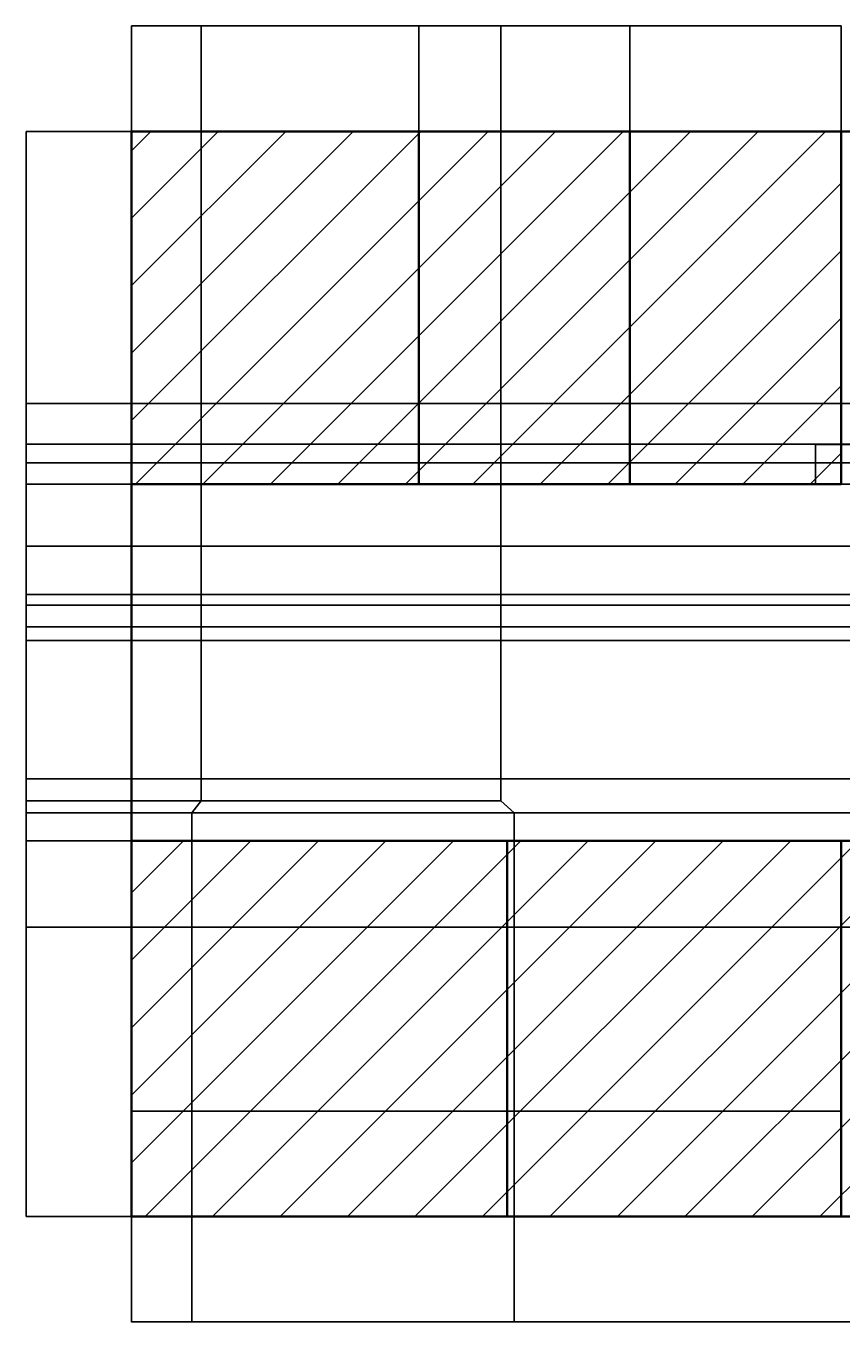
# Model space of a CAD drawing. Units: millimetres. Extents: x 2212 to 7718, y 1114 to 4219.
# Tile 1 of 5: x 2212 to 4165, y 1114 to 4219. Entities that reach past the tile are written whole.
import ezdxf

# ---------------------------------------------------------------- set-up
doc = ezdxf.new("R2010")
doc.units = ezdxf.units.MM
for name, color, linetype, lineweight in [('A-ANNO-DIMS', 2, 'Continuous', 18), ('A-ELEV-PATT', 8, 'Continuous', 13), ('A-FLOR-FIXT', 3, 'Continuous', 25), ('A-FURN', 7, 'Continuous', 35), ('A-FURN-CTOP', 6, 'Continuous', 25)]:
    doc.layers.add(name, color=color, linetype=linetype, lineweight=lineweight)
doc.styles.get("Standard").update_dxf_attribs({"font": 'arial.ttf'})
doc.dimstyles.get("Standard").update_dxf_attribs({"dimtxt": 0.18, "dimasz": 0.18, "dimexe": 0.18, "dimexo": 0.0625, "dimgap": 0.09, "dimtad": 0, "dimtih": 1, "dimtoh": 1, "dimdec": 4, "dimzin": 0, "dimdsep": 46, "dimtxsty": 'Standard', "dimcen": 0.09, "dimadec": 0, "dimazin": 0, "dimtfac": 1, "dimtdec": 4, "dimtofl": 0, "dimtmove": 0, "dimatfit": 3, "dimfxl": 1, "dimtolj": 1, "dimtzin": 0, "dimarcsym": 0})

# ---------------------------------------------------------------- blocks, each defined once
blk = doc.blocks.new('*D1')
at = {"layer": 'A-ANNO-DIMS', "color": 0, "lineweight": -2, "transparency": 16777216}
for p, q in [((2465.1, 3966.2), (2465.1, 4218.9)), ((2465.3, 4218.7), (2808.9, 4218.7)), ((3153.3, 4218.7), (2809.7, 4218.7)), ((3153.5, 3966.2), (3153.5, 4218.9))]:
    blk.add_line(p, q, dxfattribs=at)
at = {"layer": 'A-ANNO-DIMS', "color": 0, "transparency": 16777216}
for points in [[(2465.3, 4218.7), (2465.3, 4218.7), (2465.1, 4218.7)], [(3153.3, 4218.7), (3153.3, 4218.7), (3153.5, 4218.7)]]:
    blk.add_solid(points, dxfattribs=at)
at = {"layer": 'Defpoints', "color": 0, "transparency": 16777216}
for p in [(3153.5, 4218.7), (2465.1, 3966.2), (3153.5, 3966.2)]:
    blk.add_point(p, dxfattribs=at)
at = {"layer": 'A-ANNO-DIMS', "color": 0, "transparency": 16777216, "insert": (2809.3, 4218.7), "char_height": 0.18, "attachment_point": 5}
blk.add_mtext('\\A1;688.3', dxfattribs=at)
blk = doc.blocks.new('*D2')
at = {"layer": 'A-ANNO-DIMS', "color": 0, "lineweight": -2, "transparency": 16777216}
for p, q in [((3153.5, 3966.2), (3153.5, 4218.9)), ((3153.6, 4218.7), (3406, 4218.7)), ((3659.1, 4218.7), (3406.8, 4218.7)), ((3659.3, 3966.2), (3659.3, 4218.9))]:
    blk.add_line(p, q, dxfattribs=at)
at = {"layer": 'A-ANNO-DIMS', "color": 0, "transparency": 16777216}
for points in [[(3153.6, 4218.7), (3153.6, 4218.7), (3153.5, 4218.7)], [(3659.1, 4218.7), (3659.1, 4218.7), (3659.3, 4218.7)]]:
    blk.add_solid(points, dxfattribs=at)
at = {"layer": 'Defpoints', "color": 0, "transparency": 16777216}
for p in [(3659.3, 4218.7), (3153.5, 3966.2), (3659.3, 3966.2)]:
    blk.add_point(p, dxfattribs=at)
at = {"layer": 'A-ANNO-DIMS', "color": 0, "transparency": 16777216, "insert": (3406.4, 4218.7), "char_height": 0.18, "attachment_point": 5}
blk.add_mtext('\\A1;505.8', dxfattribs=at)
blk = doc.blocks.new('*D3')
at = {"layer": 'A-ANNO-DIMS', "color": 0, "lineweight": -2, "transparency": 16777216}
for p, q in [((3659.3, 3966.2), (3659.3, 4218.9)), ((3659.5, 4218.7), (3911.8, 4218.7)), ((4165, 4218.7), (3912.6, 4218.7)), ((4165.1, 3966.2), (4165.1, 4218.9))]:
    blk.add_line(p, q, dxfattribs=at)
at = {"layer": 'A-ANNO-DIMS', "color": 0, "transparency": 16777216}
for points in [[(3659.5, 4218.7), (3659.5, 4218.7), (3659.3, 4218.7)], [(4165, 4218.7), (4165, 4218.7), (4165.1, 4218.7)]]:
    blk.add_solid(points, dxfattribs=at)
at = {"layer": 'Defpoints', "color": 0, "transparency": 16777216}
for p in [(4165.1, 4218.7), (3659.3, 3966.2), (4165.1, 3966.2)]:
    blk.add_point(p, dxfattribs=at)
at = {"layer": 'A-ANNO-DIMS', "color": 0, "transparency": 16777216, "insert": (3912.2, 4218.7), "char_height": 0.18, "attachment_point": 5}
blk.add_mtext('\\A1;505.8', dxfattribs=at)
blk = doc.blocks.new('*D12')
at = {"layer": 'A-ANNO-DIMS', "color": 0, "lineweight": -2, "transparency": 16777216}
for p, q in [((4356.7, 3216.4), (4104, 3216.4)), ((4104.2, 3216.2), (4104.2, 3169)), ((4104.2, 3121.5), (4104.2, 3168.7)), ((4356.7, 3121.3), (4104, 3121.3))]:
    blk.add_line(p, q, dxfattribs=at)
at = {"layer": 'A-ANNO-DIMS', "color": 0, "transparency": 16777216}
for points in [[(4104.2, 3216.2), (4104.2, 3216.2), (4104.2, 3216.4)], [(4104.2, 3121.5), (4104.2, 3121.5), (4104.2, 3121.3)]]:
    blk.add_solid(points, dxfattribs=at)
at = {"layer": 'Defpoints', "color": 0, "transparency": 16777216}
for p in [(4104.2, 3216.4), (4356.7, 3216.4), (4356.7, 3121.3)]:
    blk.add_point(p, dxfattribs=at)
at = {"layer": 'A-ANNO-DIMS', "color": 0, "transparency": 16777216, "insert": (4104.2, 3168.9), "char_height": 0.18, "attachment_point": 5}
blk.add_mtext('\\A1;95.06', dxfattribs=at)
blk = doc.blocks.new('*D13')
at = {"layer": 'A-ANNO-DIMS', "color": 0, "lineweight": -2, "transparency": 16777216}
for p, q in [((2465.1, 1366.2), (2465.1, 1618.9)), ((2465.3, 1618.7), (2914.9, 1618.7)), ((3365, 1618.7), (2915.4, 1618.7)), ((3365.1, 1366.2), (3365.1, 1618.9))]:
    blk.add_line(p, q, dxfattribs=at)
at = {"layer": 'A-ANNO-DIMS', "color": 0, "transparency": 16777216}
for points in [[(2465.3, 1618.7), (2465.3, 1618.7), (2465.1, 1618.7)], [(3365, 1618.7), (3365, 1618.7), (3365.1, 1618.7)]]:
    blk.add_solid(points, dxfattribs=at)
at = {"layer": 'Defpoints', "color": 0, "transparency": 16777216}
for p in [(3365.1, 1618.7), (2465.1, 1366.2), (3365.1, 1366.2)]:
    blk.add_point(p, dxfattribs=at)
at = {"layer": 'A-ANNO-DIMS', "color": 0, "transparency": 16777216, "insert": (2915.1, 1618.7), "char_height": 0.18, "attachment_point": 5}
blk.add_mtext('\\A1;900', dxfattribs=at)
blk = doc.blocks.new('*D14')
at = {"layer": 'A-ANNO-DIMS', "color": 0, "lineweight": -2, "transparency": 16777216}
for p, q in [((3365.1, 1366.2), (3365.1, 1618.9)), ((3365.3, 1618.7), (3764.9, 1618.7)), ((4165, 1618.7), (3765.4, 1618.7)), ((4165.1, 1366.2), (4165.1, 1618.9))]:
    blk.add_line(p, q, dxfattribs=at)
at = {"layer": 'A-ANNO-DIMS', "color": 0, "transparency": 16777216}
for points in [[(3365.3, 1618.7), (3365.3, 1618.7), (3365.1, 1618.7)], [(4165, 1618.7), (4165, 1618.7), (4165.1, 1618.7)]]:
    blk.add_solid(points, dxfattribs=at)
at = {"layer": 'Defpoints', "color": 0, "transparency": 16777216}
for p in [(4165.1, 1618.7), (3365.1, 1366.2), (4165.1, 1366.2)]:
    blk.add_point(p, dxfattribs=at)
at = {"layer": 'A-ANNO-DIMS', "color": 0, "transparency": 16777216, "insert": (3765.1, 1618.7), "char_height": 0.18, "attachment_point": 5}
blk.add_mtext('\\A1;800', dxfattribs=at)
blk = doc.blocks.new('*D18')
at = {"layer": 'A-ANNO-DIMS', "color": 0, "lineweight": -2, "transparency": 16777216}
for p, q in [((2465.1, 1366.1), (2465.1, 1113.5)), ((7465.1, 1366.1), (7465.1, 1113.5)), ((2465.3, 1113.7), (4964.8, 1113.7)), ((7465, 1113.7), (4965.5, 1113.7))]:
    blk.add_line(p, q, dxfattribs=at)
at = {"layer": 'A-ANNO-DIMS', "color": 0, "transparency": 16777216}
for points in [[(2465.3, 1113.7), (2465.3, 1113.7), (2465.1, 1113.7)], [(7465, 1113.7), (7465, 1113.7), (7465.1, 1113.7)]]:
    blk.add_solid(points, dxfattribs=at)
at = {"layer": 'Defpoints', "color": 0, "transparency": 16777216}
for p in [(2465.1, 1366.2), (7465.1, 1366.2), (7465.1, 1113.7)]:
    blk.add_point(p, dxfattribs=at)
at = {"layer": 'A-ANNO-DIMS', "color": 0, "transparency": 16777216, "insert": (4965.1, 1113.7), "char_height": 0.18, "attachment_point": 5}
blk.add_mtext('\\A1;5000', dxfattribs=at)
blk = doc.blocks.new('*D19')
at = {"layer": 'A-ANNO-DIMS', "color": 0, "lineweight": -2, "transparency": 16777216}
for p, q in [((2465.1, 2266.4), (2212.5, 2266.4)), ((2212.6, 2266.2), (2212.6, 1816.5)), ((2212.6, 1366.4), (2212.6, 1816.1)), ((2465.1, 1366.2), (2212.5, 1366.2))]:
    blk.add_line(p, q, dxfattribs=at)
at = {"layer": 'A-ANNO-DIMS', "color": 0, "transparency": 16777216}
for points in [[(2212.6, 2266.2), (2212.7, 2266.2), (2212.6, 2266.4)], [(2212.6, 1366.4), (2212.7, 1366.4), (2212.6, 1366.2)]]:
    blk.add_solid(points, dxfattribs=at)
at = {"layer": 'Defpoints', "color": 0, "transparency": 16777216}
for p in [(2212.6, 2266.4), (2465.1, 2266.4), (2465.1, 1366.2)]:
    blk.add_point(p, dxfattribs=at)
at = {"layer": 'A-ANNO-DIMS', "color": 0, "transparency": 16777216, "insert": (2212.6, 1816.3), "char_height": 0.18, "attachment_point": 5}
blk.add_mtext('\\A1;900.2', dxfattribs=at)
blk = doc.blocks.new('*D20')
at = {"layer": 'A-ANNO-DIMS', "color": 0, "lineweight": -2, "transparency": 16777216}
for p, q in [((2465.1, 2333.4), (2212.5, 2333.4)), ((2212.6, 2333.2), (2212.6, 2300.1)), ((2212.6, 2266.6), (2212.6, 2299.7)), ((2465.1, 2266.4), (2212.5, 2266.4))]:
    blk.add_line(p, q, dxfattribs=at)
at = {"layer": 'A-ANNO-DIMS', "color": 0, "transparency": 16777216}
for points in [[(2212.6, 2333.2), (2212.7, 2333.2), (2212.6, 2333.4)], [(2212.6, 2266.6), (2212.7, 2266.6), (2212.6, 2266.4)]]:
    blk.add_solid(points, dxfattribs=at)
at = {"layer": 'Defpoints', "color": 0, "transparency": 16777216}
for p in [(2212.6, 2333.4), (2465.1, 2333.4), (2465.1, 2266.4)]:
    blk.add_point(p, dxfattribs=at)
at = {"layer": 'A-ANNO-DIMS', "color": 0, "transparency": 16777216, "insert": (2212.6, 2299.9), "char_height": 0.18, "attachment_point": 5}
blk.add_mtext('\\A1;66.97', dxfattribs=at)
blk = doc.blocks.new('*D21')
at = {"layer": 'A-ANNO-DIMS', "color": 0, "lineweight": -2, "transparency": 16777216}
for p, q in [((2465.1, 2414.8), (2212.5, 2414.8)), ((2212.6, 2414.6), (2212.6, 2374.3)), ((2212.6, 2333.5), (2212.6, 2373.9)), ((2465.1, 2333.4), (2212.5, 2333.4))]:
    blk.add_line(p, q, dxfattribs=at)
at = {"layer": 'A-ANNO-DIMS', "color": 0, "transparency": 16777216}
for points in [[(2212.6, 2414.6), (2212.7, 2414.6), (2212.6, 2414.8)], [(2212.6, 2333.5), (2212.7, 2333.5), (2212.6, 2333.4)]]:
    blk.add_solid(points, dxfattribs=at)
at = {"layer": 'Defpoints', "color": 0, "transparency": 16777216}
for p in [(2212.6, 2414.8), (2465.1, 2414.8), (2465.1, 2333.4)]:
    blk.add_point(p, dxfattribs=at)
at = {"layer": 'A-ANNO-DIMS', "color": 0, "transparency": 16777216, "insert": (2212.6, 2374.1), "char_height": 0.18, "attachment_point": 5}
blk.add_mtext('\\A1;81.45', dxfattribs=at)
blk = doc.blocks.new('*D22')
at = {"layer": 'A-ANNO-DIMS', "color": 0, "lineweight": -2, "transparency": 16777216}
for p, q in [((2465.1, 3121.3), (2212.5, 3121.3)), ((2212.6, 3121.2), (2212.6, 2768.3)), ((2212.6, 2415), (2212.6, 2767.9)), ((2465.1, 2414.8), (2212.5, 2414.8))]:
    blk.add_line(p, q, dxfattribs=at)
at = {"layer": 'A-ANNO-DIMS', "color": 0, "transparency": 16777216}
for points in [[(2212.6, 3121.2), (2212.7, 3121.2), (2212.6, 3121.3)], [(2212.6, 2415), (2212.7, 2415), (2212.6, 2414.8)]]:
    blk.add_solid(points, dxfattribs=at)
at = {"layer": 'Defpoints', "color": 0, "transparency": 16777216}
for p in [(2212.6, 3121.3), (2465.1, 3121.3), (2465.1, 2414.8)]:
    blk.add_point(p, dxfattribs=at)
at = {"layer": 'A-ANNO-DIMS', "color": 0, "transparency": 16777216, "insert": (2212.6, 2768.1), "char_height": 0.18, "attachment_point": 5}
blk.add_mtext('\\A1;706.5', dxfattribs=at)
blk = doc.blocks.new('*D23')
at = {"layer": 'A-ANNO-DIMS', "color": 0, "lineweight": -2, "transparency": 16777216}
for p, q in [((2465.1, 3966.2), (2212.5, 3966.2)), ((2212.6, 3966), (2212.6, 3543.9)), ((2212.6, 3121.5), (2212.6, 3543.6)), ((2465.1, 3121.3), (2212.5, 3121.3))]:
    blk.add_line(p, q, dxfattribs=at)
at = {"layer": 'A-ANNO-DIMS', "color": 0, "transparency": 16777216}
for points in [[(2212.6, 3966), (2212.7, 3966), (2212.6, 3966.2)], [(2212.6, 3121.5), (2212.7, 3121.5), (2212.6, 3121.3)]]:
    blk.add_solid(points, dxfattribs=at)
at = {"layer": 'Defpoints', "color": 0, "transparency": 16777216}
for p in [(2212.6, 3966.2), (2465.1, 3966.2), (2465.1, 3121.3)]:
    blk.add_point(p, dxfattribs=at)
at = {"layer": 'A-ANNO-DIMS', "color": 0, "transparency": 16777216, "insert": (2212.6, 3543.8), "char_height": 0.18, "attachment_point": 5}
blk.add_mtext('\\A1;844.8', dxfattribs=at)
blk = doc.blocks.new('*D27')
at = {"layer": 'A-ANNO-DIMS', "color": 0, "lineweight": -2, "transparency": 16777216}
for p, q in [((5865.1, 2746.8), (2212.5, 2746.8)), ((2212.6, 2746.6), (2212.6, 2403.4)), ((2212.6, 2059.8), (2212.6, 2403)), ((5865.1, 2059.6), (2212.5, 2059.6))]:
    blk.add_line(p, q, dxfattribs=at)
at = {"layer": 'A-ANNO-DIMS', "color": 0, "transparency": 16777216}
for points in [[(2212.6, 2746.6), (2212.7, 2746.6), (2212.6, 2746.8)], [(2212.6, 2059.8), (2212.7, 2059.8), (2212.6, 2059.6)]]:
    blk.add_solid(points, dxfattribs=at)
at = {"layer": 'Defpoints', "color": 0, "transparency": 16777216}
for p in [(2212.6, 2746.8), (5865.1, 2746.8), (5865.1, 2059.6)]:
    blk.add_point(p, dxfattribs=at)
at = {"layer": 'A-ANNO-DIMS', "color": 0, "transparency": 16777216, "insert": (2212.6, 2403.2), "char_height": 0.18, "attachment_point": 5}
blk.add_mtext('\\A1;687.2', dxfattribs=at)
blk = doc.blocks.new('*D28')
at = {"layer": 'A-ANNO-DIMS', "color": 0, "lineweight": -2, "transparency": 16777216}
for p, q in [((5865.1, 2856.7), (2212.5, 2856.7)), ((2212.6, 2856.6), (2212.6, 2802)), ((2212.6, 2747), (2212.6, 2801.6)), ((5865.1, 2746.8), (2212.5, 2746.8))]:
    blk.add_line(p, q, dxfattribs=at)
at = {"layer": 'A-ANNO-DIMS', "color": 0, "transparency": 16777216}
for points in [[(2212.6, 2856.6), (2212.7, 2856.6), (2212.6, 2856.7)], [(2212.6, 2747), (2212.7, 2747), (2212.6, 2746.8)]]:
    blk.add_solid(points, dxfattribs=at)
at = {"layer": 'Defpoints', "color": 0, "transparency": 16777216}
for p in [(2212.6, 2856.7), (5865.1, 2856.7), (5865.1, 2746.8)]:
    blk.add_point(p, dxfattribs=at)
at = {"layer": 'A-ANNO-DIMS', "color": 0, "transparency": 16777216, "insert": (2212.6, 2801.8), "char_height": 0.18, "attachment_point": 5}
blk.add_mtext('\\A1;109.95', dxfattribs=at)
blk = doc.blocks.new('*D29')
at = {"layer": 'A-ANNO-DIMS', "color": 0, "lineweight": -2, "transparency": 16777216}
for p, q in [((5865.1, 3217.2), (2212.5, 3217.2)), ((2212.6, 3217.1), (2212.6, 3037.2)), ((2212.6, 2856.9), (2212.6, 3036.8)), ((5865.1, 2856.7), (2212.5, 2856.7))]:
    blk.add_line(p, q, dxfattribs=at)
at = {"layer": 'A-ANNO-DIMS', "color": 0, "transparency": 16777216}
for points in [[(2212.6, 3217.1), (2212.7, 3217.1), (2212.6, 3217.2)], [(2212.6, 2856.9), (2212.7, 2856.9), (2212.6, 2856.7)]]:
    blk.add_solid(points, dxfattribs=at)
at = {"layer": 'Defpoints', "color": 0, "transparency": 16777216}
for p in [(2212.6, 3217.2), (5865.1, 3217.2), (5865.1, 2856.7)]:
    blk.add_point(p, dxfattribs=at)
at = {"layer": 'A-ANNO-DIMS', "color": 0, "transparency": 16777216, "insert": (2212.6, 3037), "char_height": 0.18, "attachment_point": 5}
blk.add_mtext('\\A1;360.5', dxfattribs=at)
blk = doc.blocks.new('*D30')
at = {"layer": 'A-ANNO-DIMS', "color": 0, "lineweight": -2, "transparency": 16777216}
for p, q in [((5865.1, 3314.4), (2212.5, 3314.4)), ((2212.6, 3314.2), (2212.6, 3266)), ((2212.6, 3217.4), (2212.6, 3265.6)), ((5865.1, 3217.2), (2212.5, 3217.2))]:
    blk.add_line(p, q, dxfattribs=at)
at = {"layer": 'A-ANNO-DIMS', "color": 0, "transparency": 16777216}
for points in [[(2212.6, 3314.2), (2212.7, 3314.2), (2212.6, 3314.4)], [(2212.6, 3217.4), (2212.7, 3217.4), (2212.6, 3217.2)]]:
    blk.add_solid(points, dxfattribs=at)
at = {"layer": 'Defpoints', "color": 0, "transparency": 16777216}
for p in [(2212.6, 3314.4), (5865.1, 3314.4), (5865.1, 3217.2)]:
    blk.add_point(p, dxfattribs=at)
at = {"layer": 'A-ANNO-DIMS', "color": 0, "transparency": 16777216, "insert": (2212.6, 3265.8), "char_height": 0.18, "attachment_point": 5}
blk.add_mtext('\\A1;97.14', dxfattribs=at)
blk = doc.blocks.new('*D31')
at = {"layer": 'A-ANNO-DIMS', "color": 0, "lineweight": -2, "transparency": 16777216}
for p, q in [((5865.1, 3966.2), (2212.5, 3966.2)), ((2212.6, 3966), (2212.6, 3640.5)), ((2212.6, 3314.6), (2212.6, 3640.1)), ((5865.1, 3314.4), (2212.5, 3314.4))]:
    blk.add_line(p, q, dxfattribs=at)
at = {"layer": 'A-ANNO-DIMS', "color": 0, "transparency": 16777216}
for points in [[(2212.6, 3966), (2212.7, 3966), (2212.6, 3966.2)], [(2212.6, 3314.6), (2212.7, 3314.6), (2212.6, 3314.4)]]:
    blk.add_solid(points, dxfattribs=at)
at = {"layer": 'Defpoints', "color": 0, "transparency": 16777216}
for p in [(2212.6, 3966.2), (5865.1, 3966.2), (5865.1, 3314.4)]:
    blk.add_point(p, dxfattribs=at)
at = {"layer": 'A-ANNO-DIMS', "color": 0, "transparency": 16777216, "insert": (2212.6, 3640.3), "char_height": 0.18, "attachment_point": 5}
blk.add_mtext('\\A1;651.8', dxfattribs=at)
blk = doc.blocks.new('*D37')
at = {"layer": 'A-ANNO-DIMS', "color": 0, "lineweight": -2, "transparency": 16777216}
for p, q in [((6027.7, 2972.2), (2212.5, 2972.2)), ((2212.6, 2972), (2212.6, 2914.6)), ((2212.6, 2856.9), (2212.6, 2914.3)), ((5930.4, 2856.7), (2212.5, 2856.7))]:
    blk.add_line(p, q, dxfattribs=at)
at = {"layer": 'A-ANNO-DIMS', "color": 0, "transparency": 16777216}
for points in [[(2212.6, 2972), (2212.7, 2972), (2212.6, 2972.2)], [(2212.6, 2856.9), (2212.7, 2856.9), (2212.6, 2856.7)]]:
    blk.add_solid(points, dxfattribs=at)
at = {"layer": 'Defpoints', "color": 0, "transparency": 16777216}
for p in [(2212.6, 2972.2), (6027.8, 2972.2), (5930.5, 2856.7)]:
    blk.add_point(p, dxfattribs=at)
at = {"layer": 'A-ANNO-DIMS', "color": 0, "transparency": 16777216, "insert": (2212.6, 2914.5), "char_height": 0.18, "attachment_point": 5}
blk.add_mtext('\\A1;115.44', dxfattribs=at)
blk = doc.blocks.new('*D42')
at = {"layer": 'A-ANNO-DIMS', "color": 0, "lineweight": -2, "transparency": 16777216}
for p, q in [((6506, 3217.2), (2212.5, 3217.2)), ((2212.6, 3217.1), (2212.6, 3195)), ((6530.4, 3172.4), (2212.5, 3172.4)), ((2212.6, 3172.6), (2212.6, 3194.6))]:
    blk.add_line(p, q, dxfattribs=at)
at = {"layer": 'A-ANNO-DIMS', "color": 0, "transparency": 16777216}
for points in [[(2212.6, 3217.1), (2212.7, 3217.1), (2212.6, 3217.2)], [(2212.6, 3172.6), (2212.7, 3172.6), (2212.6, 3172.4)]]:
    blk.add_solid(points, dxfattribs=at)
at = {"layer": 'Defpoints', "color": 0, "transparency": 16777216}
for p in [(6506.1, 3217.2), (2212.6, 3172.4), (6530.5, 3172.4)]:
    blk.add_point(p, dxfattribs=at)
at = {"layer": 'A-ANNO-DIMS', "color": 0, "transparency": 16777216, "insert": (2212.6, 3194.8), "char_height": 0.18, "attachment_point": 5}
blk.add_mtext('\\A1;44.855', dxfattribs=at)
blk = doc.blocks.new('*D44')
at = {"layer": 'A-ANNO-DIMS', "color": 0, "lineweight": -2, "transparency": 16777216}
for p, q in [((6023.8, 2830.9), (2212.5, 2830.9)), ((2212.6, 2830.7), (2212.6, 2805.3)), ((2212.6, 2779.5), (2212.6, 2804.9)), ((6023.8, 2779.3), (2212.5, 2779.3))]:
    blk.add_line(p, q, dxfattribs=at)
at = {"layer": 'A-ANNO-DIMS', "color": 0, "transparency": 16777216}
for points in [[(2212.6, 2830.7), (2212.7, 2830.7), (2212.6, 2830.9)], [(2212.6, 2779.5), (2212.7, 2779.5), (2212.6, 2779.3)]]:
    blk.add_solid(points, dxfattribs=at)
at = {"layer": 'Defpoints', "color": 0, "transparency": 16777216}
for p in [(2212.6, 2830.9), (6023.9, 2830.9), (6023.9, 2779.3)]:
    blk.add_point(p, dxfattribs=at)
at = {"layer": 'A-ANNO-DIMS', "color": 0, "transparency": 16777216, "insert": (2212.6, 2805.1), "char_height": 0.18, "attachment_point": 5}
blk.add_mtext('\\A1;51.58', dxfattribs=at)
blk = doc.blocks.new('*D57')
at = {"layer": 'A-ANNO-DIMS', "color": 0, "lineweight": -2, "transparency": 16777216}
for p, q in [((2465.1, 2333.3), (2465.1, 1113.5)), ((2609.9, 2333.3), (2609.9, 1113.5)), ((2465.3, 1113.7), (2537.1, 1113.7)), ((2609.7, 1113.7), (2538, 1113.7))]:
    blk.add_line(p, q, dxfattribs=at)
at = {"layer": 'A-ANNO-DIMS', "color": 0, "transparency": 16777216}
for points in [[(2465.3, 1113.7), (2465.3, 1113.7), (2465.1, 1113.7)], [(2609.7, 1113.7), (2609.7, 1113.7), (2609.9, 1113.7)]]:
    blk.add_solid(points, dxfattribs=at)
at = {"layer": 'Defpoints', "color": 0, "transparency": 16777216}
for p in [(2465.1, 2333.4), (2609.9, 2333.4), (2609.9, 1113.7)]:
    blk.add_point(p, dxfattribs=at)
at = {"layer": 'A-ANNO-DIMS', "color": 0, "transparency": 16777216, "insert": (2537.5, 1113.7), "char_height": 0.18, "attachment_point": 5}
blk.add_mtext('\\A1;144.78', dxfattribs=at)
blk = doc.blocks.new('*D58')
at = {"layer": 'A-ANNO-DIMS', "color": 0, "lineweight": -2, "transparency": 16777216}
for p, q in [((2609.9, 2333.3), (2609.9, 1113.5)), ((3382, 2333.3), (3382, 1113.5)), ((2610.1, 1113.7), (2995.5, 1113.7)), ((3381.9, 1113.7), (2996.4, 1113.7))]:
    blk.add_line(p, q, dxfattribs=at)
at = {"layer": 'A-ANNO-DIMS', "color": 0, "transparency": 16777216}
for points in [[(2610.1, 1113.7), (2610.1, 1113.7), (2609.9, 1113.7)], [(3381.9, 1113.7), (3381.9, 1113.7), (3382, 1113.7)]]:
    blk.add_solid(points, dxfattribs=at)
at = {"layer": 'Defpoints', "color": 0, "transparency": 16777216}
for p in [(2609.9, 2333.4), (3382, 2333.4), (3382, 1113.7)]:
    blk.add_point(p, dxfattribs=at)
at = {"layer": 'A-ANNO-DIMS', "color": 0, "transparency": 16777216, "insert": (2996, 1113.7), "char_height": 0.18, "attachment_point": 5}
blk.add_mtext('\\A1;772.12', dxfattribs=at)
blk = doc.blocks.new('*D59')
at = {"layer": 'A-ANNO-DIMS', "color": 0, "lineweight": -2, "transparency": 16777216}
for p, q in [((2632.2, 2362.7), (2632.2, 4218.9)), ((2632.4, 4218.7), (2990.6, 4218.7)), ((3349.8, 4218.7), (2991.6, 4218.7)), ((3350, 2362.7), (3350, 4218.9))]:
    blk.add_line(p, q, dxfattribs=at)
at = {"layer": 'A-ANNO-DIMS', "color": 0, "transparency": 16777216}
for points in [[(2632.4, 4218.7), (2632.4, 4218.7), (2632.2, 4218.7)], [(3349.8, 4218.7), (3349.8, 4218.7), (3350, 4218.7)]]:
    blk.add_solid(points, dxfattribs=at)
at = {"layer": 'Defpoints', "color": 0, "transparency": 16777216}
for p in [(3350, 4218.7), (2632.2, 2362.6), (3350, 2362.6)]:
    blk.add_point(p, dxfattribs=at)
at = {"layer": 'A-ANNO-DIMS', "color": 0, "transparency": 16777216, "insert": (2991.1, 4218.7), "char_height": 0.18, "attachment_point": 5}
blk.add_mtext('\\A1;717.77', dxfattribs=at)
blk = doc.blocks.new('*D60')
at = {"layer": 'A-ANNO-DIMS', "color": 0, "lineweight": -2, "transparency": 16777216}
for p, q in [((2465.1, 2333.4), (2465.1, 4218.9)), ((2465.3, 4218.7), (2548.2, 4218.7)), ((2632, 4218.7), (2549.1, 4218.7)), ((2632.2, 2362.7), (2632.2, 4218.9))]:
    blk.add_line(p, q, dxfattribs=at)
at = {"layer": 'A-ANNO-DIMS', "color": 0, "transparency": 16777216}
for points in [[(2465.3, 4218.7), (2465.3, 4218.7), (2465.1, 4218.7)], [(2632, 4218.7), (2632, 4218.7), (2632.2, 4218.7)]]:
    blk.add_solid(points, dxfattribs=at)
at = {"layer": 'Defpoints', "color": 0, "transparency": 16777216}
for p in [(2632.2, 4218.7), (2632.2, 2362.6), (2465.1, 2333.4)]:
    blk.add_point(p, dxfattribs=at)
at = {"layer": 'A-ANNO-DIMS', "color": 0, "transparency": 16777216, "insert": (2548.7, 4218.7), "char_height": 0.18, "attachment_point": 5}
blk.add_mtext('\\A1;167.08', dxfattribs=at)
blk = doc.blocks.new('*D61')
at = {"layer": 'A-ANNO-DIMS', "color": 0, "lineweight": -2, "transparency": 16777216}
for p, q in [((2632.2, 2362.6), (2212.5, 2362.6)), ((2212.6, 2362.4), (2212.6, 2348.2)), ((2609.9, 2333.4), (2212.5, 2333.4)), ((2212.6, 2333.5), (2212.6, 2347.8))]:
    blk.add_line(p, q, dxfattribs=at)
at = {"layer": 'A-ANNO-DIMS', "color": 0, "transparency": 16777216}
for points in [[(2212.6, 2362.4), (2212.7, 2362.4), (2212.6, 2362.6)], [(2212.6, 2333.5), (2212.7, 2333.5), (2212.6, 2333.4)]]:
    blk.add_solid(points, dxfattribs=at)
at = {"layer": 'Defpoints', "color": 0, "transparency": 16777216}
for p in [(2212.6, 2362.6), (2632.2, 2362.6), (2609.9, 2333.4)]:
    blk.add_point(p, dxfattribs=at)
at = {"layer": 'A-ANNO-DIMS', "color": 0, "transparency": 16777216, "insert": (2212.6, 2348), "char_height": 0.18, "attachment_point": 5}
blk.add_mtext('\\A1;29.23', dxfattribs=at)

msp = doc.modelspace()

# ---------------------------------------------------------------- hatches: boundary and pattern name
at = {"layer": 'A-ELEV-PATT'}
h = msp.add_hatch(dxfattribs=at)
h.set_pattern_fill('ANSI31', color=256, scale=36)
h.paths.add_polyline_path([(3153.454, 3966.1829), (2465.1412, 3966.1829), (2465.1412, 3121.3339), (3153.454, 3121.3339)])
h.paths.add_polyline_path([(3659.2976, 3966.1829), (3153.454, 3966.1829), (3153.454, 3121.3339), (3659.2976, 3121.3339)])
h.paths.add_polyline_path([(4165.1412, 3966.1829), (3659.2976, 3966.1829), (3659.2976, 3121.3339), (4165.1412, 3121.3339)])
h.paths.add_polyline_path([(3365.1412, 2266.3983), (2465.1412, 2266.3983), (2465.1412, 1366.1829), (3365.1412, 1366.1829)])
h.paths.add_polyline_path([(4165.1412, 2266.3983), (3365.1412, 2266.3983), (3365.1412, 1366.1829), (4165.1412, 1366.1829)])
h.paths.add_polyline_path([(4965.1412, 2266.3983), (4165.1412, 2266.3983), (4165.1412, 1366.1829), (4965.1412, 1366.1829)])
h.paths.add_polyline_path([(5765.1412, 2266.3983), (4965.1412, 2266.3983), (4965.1412, 1366.1829), (5765.1412, 1366.1829)])
h.paths.add_polyline_path([(6665.1412, 2059.6125), (5865.1412, 2059.6125), (5865.1412, 1366.1829), (6665.1412, 1366.1829)])
h.paths.add_polyline_path([(7465.1412, 2266.3983), (7065.1412, 2266.3983), (7065.1412, 1366.1829), (7465.1412, 1366.1829)])
h.paths.add_polyline_path([(7065.1412, 2266.3983), (6665.1412, 2266.3983), (6665.1412, 1366.1829), (7065.1412, 1366.1829)])
h.paths.add_polyline_path([(7465.1412, 3966.1829), (7065.1412, 3966.1829), (7065.1412, 2266.3983), (7465.1412, 2266.3983)])
h.paths.add_polyline_path([(7065.1412, 3966.1829), (6665.1412, 3966.1829), (6665.1412, 2266.3983), (7065.1412, 2266.3983)])
h.paths.add_polyline_path([(6665.1412, 3966.1829), (6027.7806, 3966.1829), (6027.7806, 3314.3715), (6665.1412, 3314.3715)])
h.paths.add_polyline_path([(5245.7331, 3966.1829), (4821.5849, 3966.1829), (4821.5849, 3216.3983), (4356.7186, 3216.3983), (4356.7186, 3121.3339), (5503.6152, 3121.3339), (5720.779, 3121.3339), (5720.779, 3216.3983), (5245.7331, 3216.3983)])

# ---------------------------------------------------------------- linework, layer by layer
at = {"layer": 'A-FLOR-FIXT'}
for p, q in [((2609.9176, 2333.3682), (2632.2171, 2362.5987)), ((2632.2171, 2362.5987), (3349.9851, 2362.5987)), ((3349.9851, 2362.5987), (3382.0408, 2333.3682))]:
    msp.add_line(p, q, dxfattribs=at)
at = {"layer": 'A-FURN'}
for p, q in [((2465.1412, 3966.1829), (5865.1412, 3966.1829)), ((2465.1412, 1366.1829), (2465.1412, 3966.1829)), ((3153.454, 3966.1829), (3153.454, 3121.3339)), ((3659.2976, 3121.3339), (3659.2976, 3966.1829)), ((4165.1412, 3966.1829), (4165.1412, 3121.3339)), ((3153.454, 3121.3339), (2465.1412, 3121.3339)), ((4165.1412, 3121.3339), (3153.454, 3121.3339)), ((5765.1412, 2266.3983), (2465.1412, 2266.3983)), ((3365.1412, 1366.1829), (3365.1412, 2266.3983)), ((4165.1412, 1366.1829), (4165.1412, 2266.3983)), ((5865.1412, 1366.1829), (2465.1412, 1366.1829)), ((2465.1412, 1366.1829), (3365.1412, 1366.1829)), ((3365.1412, 1366.1829), (4165.1412, 1366.1829)), ((4165.1412, 1366.1829), (4965.1412, 1366.1829))]:
    msp.add_line(p, q, dxfattribs=at)
at = {"layer": 'A-FURN-CTOP'}
for p, q in [((5865.1412, 2414.8193), (2465.1412, 2414.8193)), ((2465.1412, 2333.3682), (5865.1412, 2333.3682))]:
    msp.add_line(p, q, dxfattribs=at)

# ---------------------------------------------------------------- dimensions: what is measured, and where the dimension line sits
at = {"layer": 'A-ANNO-DIMS'}
for base, p1, p2, override, picture, middle in [((3153.454, 4218.6829), (2465.1412, 3966.1829), (3153.454, 3966.1829), {"dimdec": 1, "dimlfac": 1, "dimrnd": 0, "dimzin": 0, "dimdsep": 46, "dimlunit": 2}, '*D1', (2809.2976, 4218.6829)), ((2632.2171, 4218.6829), (2465.1412, 2333.3682), (2632.2171, 2362.5987), {"dimdec": 2, "dimlfac": 1, "dimrnd": 0, "dimzin": 0, "dimdsep": 46, "dimlunit": 2}, '*D60', (2548.6792, 4218.6829)), ((3349.9851, 4218.6829), (2632.2171, 2362.5987), (3349.9851, 2362.5987), {"dimdec": 2, "dimlfac": 1, "dimrnd": 0, "dimzin": 0, "dimdsep": 46, "dimlunit": 2}, '*D59', (2991.1011, 4218.6829)), ((3659.2976, 4218.6829), (3153.454, 3966.1829), (3659.2976, 3966.1829), {"dimdec": 1, "dimlfac": 1, "dimrnd": 0, "dimzin": 0, "dimdsep": 46, "dimlunit": 2}, '*D2', (3406.3758, 4218.6829)), ((4165.1412, 4218.6829), (3659.2976, 3966.1829), (4165.1412, 3966.1829), {"dimdec": 1, "dimlfac": 1, "dimrnd": 0, "dimzin": 0, "dimdsep": 46, "dimlunit": 2}, '*D3', (3912.2194, 4218.6829)), ((2609.9176, 1113.6829), (2465.1412, 2333.3682), (2609.9176, 2333.3682), {"dimdec": 2, "dimlfac": 1, "dimrnd": 0, "dimzin": 0, "dimdsep": 46, "dimlunit": 2}, '*D57', (2537.5294, 1113.6829)), ((3382.0408, 1113.6829), (2609.9176, 2333.3682), (3382.0408, 2333.3682), {"dimdec": 2, "dimlfac": 1, "dimrnd": 0, "dimzin": 0, "dimdsep": 46, "dimlunit": 2}, '*D58', (2995.9792, 1113.6829)), ((3365.1412, 1618.6829), (2465.1412, 1366.1829), (3365.1412, 1366.1829), {"dimdec": 0, "dimlfac": 1, "dimrnd": 0, "dimzin": 0, "dimdsep": 46, "dimlunit": 2}, '*D13', (2915.1412, 1618.6829)), ((4165.1412, 1618.6829), (3365.1412, 1366.1829), (4165.1412, 1366.1829), {"dimdec": 0, "dimlfac": 1, "dimrnd": 0, "dimzin": 0, "dimdsep": 46, "dimlunit": 2}, '*D14', (3765.1412, 1618.6829)), ((7465.1412, 1113.6829), (2465.1412, 1366.1829), (7465.1412, 1366.1829), {"dimdec": 0, "dimlfac": 1, "dimrnd": 0, "dimzin": 0, "dimdsep": 46, "dimlunit": 2}, '*D18', (4965.1412, 1113.6829))]:
    dim = msp.add_linear_dim(base=base, p1=p1, p2=p2, dimstyle='Standard', override=override, dxfattribs=at)
    dim.commit()
    dim.dimension.update_dxf_attribs({"geometry": picture, "text_midpoint": middle})
for base, p1, p2, override, picture, middle in [((2212.6412, 3966.1829), (2465.1412, 3121.3339), (2465.1412, 3966.1829), {"dimdec": 1, "dimlfac": 1, "dimrnd": 0, "dimzin": 0, "dimdsep": 46, "dimlunit": 2}, '*D23', (2212.6412, 3543.7584)), ((2212.6412, 3966.1829), (5865.1412, 3314.3715), (5865.1412, 3966.1829), {"dimdec": 1, "dimlfac": 1, "dimrnd": 0, "dimzin": 0, "dimdsep": 46, "dimlunit": 2}, '*D31', (2212.6412, 3640.2772)), ((2212.6412, 3314.3715), (5865.1412, 3217.2303), (5865.1412, 3314.3715), {"dimdec": 2, "dimlfac": 1, "dimrnd": 0, "dimzin": 0, "dimdsep": 46, "dimlunit": 2}, '*D30', (2212.6412, 3265.8009)), ((2212.6412, 3172.3755), (6506.0666, 3217.2303), (6530.4592, 3172.3755), {"dimdec": 3, "dimlfac": 1, "dimrnd": 0, "dimzin": 0, "dimdsep": 46, "dimlunit": 2}, '*D42', (2212.6412, 3194.8029)), ((2212.6412, 3217.2303), (5865.1412, 2856.7409), (5865.1412, 3217.2303), {"dimdec": 1, "dimlfac": 1, "dimrnd": 0, "dimzin": 0, "dimdsep": 46, "dimlunit": 2}, '*D29', (2212.6412, 3036.9856)), ((4104.2186, 3216.3983), (4356.7186, 3121.3339), (4356.7186, 3216.3983), {"dimdec": 2, "dimlfac": 1, "dimrnd": 0, "dimzin": 0, "dimdsep": 46, "dimlunit": 2}, '*D12', (4104.2186, 3168.8661)), ((2212.6412, 3121.3339), (2465.1412, 2414.8193), (2465.1412, 3121.3339), {"dimdec": 1, "dimlfac": 1, "dimrnd": 0, "dimzin": 0, "dimdsep": 46, "dimlunit": 2}, '*D22', (2212.6412, 2768.0766)), ((2212.6412, 2972.1846), (5930.461, 2856.7409), (6027.7806, 2972.1846), {"dimdec": 2, "dimlfac": 1, "dimrnd": 0, "dimzin": 0, "dimdsep": 46, "dimlunit": 2}, '*D37', (2212.6412, 2914.4628)), ((2212.6412, 2856.7409), (5865.1412, 2746.7954), (5865.1412, 2856.7409), {"dimdec": 2, "dimlfac": 1, "dimrnd": 0, "dimzin": 0, "dimdsep": 46, "dimlunit": 2}, '*D28', (2212.6412, 2801.7682)), ((2212.6412, 2830.8799), (6023.8866, 2779.2966), (6023.8866, 2830.8799), {"dimdec": 2, "dimlfac": 1, "dimrnd": 0, "dimzin": 0, "dimdsep": 46, "dimlunit": 2}, '*D44', (2212.6412, 2805.0882)), ((2212.6412, 2746.7954), (5865.1412, 2059.6125), (5865.1412, 2746.7954), {"dimdec": 1, "dimlfac": 1, "dimrnd": 0, "dimzin": 0, "dimdsep": 46, "dimlunit": 2}, '*D27', (2212.6412, 2403.204)), ((2212.6412, 2414.8193), (2465.1412, 2333.3682), (2465.1412, 2414.8193), {"dimdec": 2, "dimlfac": 1, "dimrnd": 0, "dimzin": 0, "dimdsep": 46, "dimlunit": 2}, '*D21', (2212.6412, 2374.0937)), ((2212.6412, 2362.5987), (2609.9176, 2333.3682), (2632.2171, 2362.5987), {"dimdec": 2, "dimlfac": 1, "dimrnd": 0, "dimzin": 0, "dimdsep": 46, "dimlunit": 2}, '*D61', (2212.6412, 2347.9835)), ((2212.6412, 2333.3682), (2465.1412, 2266.3983), (2465.1412, 2333.3682), {"dimdec": 2, "dimlfac": 1, "dimrnd": 0, "dimzin": 0, "dimdsep": 46, "dimlunit": 2}, '*D20', (2212.6412, 2299.8833)), ((2212.6412, 2266.3983), (2465.1412, 1366.1829), (2465.1412, 2266.3983), {"dimdec": 1, "dimlfac": 1, "dimrnd": 0, "dimzin": 0, "dimdsep": 46, "dimlunit": 2}, '*D19', (2212.6412, 1816.2906))]:
    dim = msp.add_linear_dim(base=base, p1=p1, p2=p2, angle=90, dimstyle='Standard', override=override, dxfattribs=at)
    dim.commit()
    dim.dimension.update_dxf_attribs({"geometry": picture, "text_midpoint": middle})

doc.saveas('drawing.dxf')
